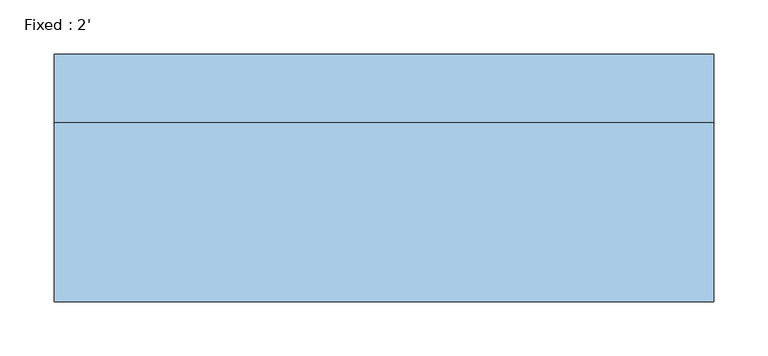
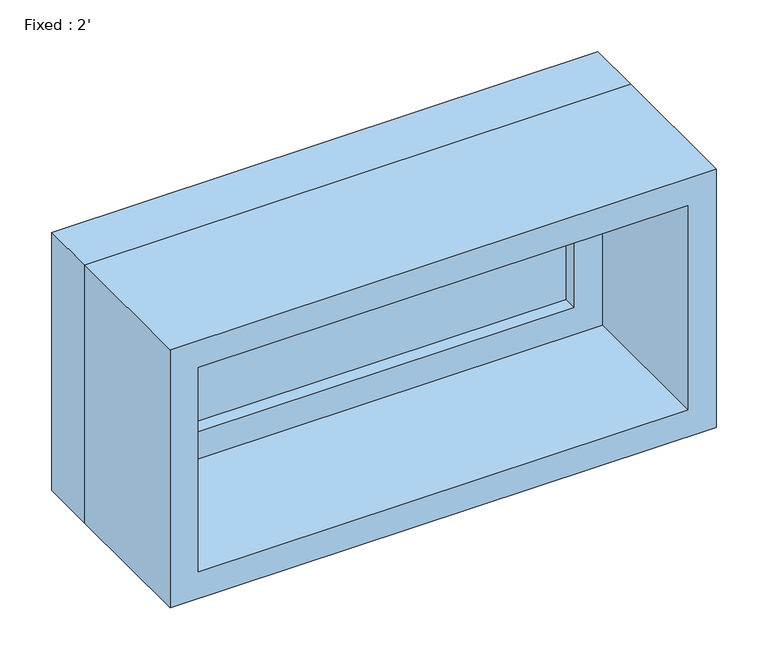
"""IFC4 building model written with IfcOpenShell, lengths in millimetres: window geometry, Fixed : 2'."""

from ifc_helpers import new_model, si_unit, frame, origin, place, context, project, spatial, polyline, outline, extrude, source, transform, mapped, element, save


def fixed_2_8c8825d0(model_context):
    return source(origin(), model_context, "Body", "SweptSolid", [
        extrude(outline(polyline([(203.2, 66.675), (-279.4, 66.675), (-279.4, 79.375), (203.2, 79.375), (203.2, 66.675)])), frame((0.0, 0.0, 977.9), z_axis=(0.0, 0.0, 1.0), x_axis=(1.0, 0.0, 0.0)), (0.0, 0.0, 1.0), 177.8),
        extrude(outline(polyline([(1200.15, -323.85), (933.45, -323.85), (933.45, 247.65), (1200.15, 247.65), (1200.15, -323.85)]), holes=[polyline([(1155.7, -279.4), (1155.7, 203.2), (977.9, 203.2), (977.9, -279.4), (1155.7, -279.4)])]), frame((0.0, 50.8, 0.0), z_axis=(0.0, 1.0, 0.0), x_axis=(0.0, 0.0, 1.0)), (0.0, 0.0, 1.0), 44.45),
        extrude(outline(polyline([(1219.2, -342.9), (914.4, -342.9), (914.4, 266.7), (1219.2, 266.7), (1219.2, -342.9)]), holes=[polyline([(1187.45, -311.15), (1187.45, 234.95), (946.15, 234.95), (946.15, -311.15), (1187.45, -311.15)])]), frame((0.0, -114.3, 0.0), z_axis=(0.0, 1.0, 0.0), x_axis=(0.0, 0.0, 1.0)), (0.0, 0.0, 1.0), 165.1),
        extrude(outline(polyline([(1219.2, 266.7), (1219.2, -342.9), (914.4, -342.9), (914.4, 266.7), (1219.2, 266.7)]), holes=[polyline([(1200.15, 247.65), (933.45, 247.65), (933.45, -323.85), (1200.15, -323.85), (1200.15, 247.65)])]), frame((0.0, 50.8, 0.0), z_axis=(0.0, 1.0, 0.0), x_axis=(0.0, 0.0, 1.0)), (0.0, 0.0, 1.0), 63.5),
    ])


if __name__ == "__main__":
    model = new_model("IFC4")
    model_context = context("Model", 3, world=origin())
    ifc_project = project(units=[si_unit("LENGTHUNIT", "METRE", prefix="MILLI")], contexts=[model_context])
    site = spatial("IfcSite", under=ifc_project)
    building = spatial("IfcBuilding", under=site)
    placement = place(None, origin())
    fixed_2_shape = fixed_2_8c8825d0(model_context)
    element("IfcWindow", 1, ObjectType="Fixed : 2'", at=placement, inside=building, context=model_context, shape_type="MappedRepresentation", body=[
        mapped(fixed_2_shape, transform((0.0, 0.0, 0.0), x_axis=(1.0, 0.0, 0.0), y_axis=(0.0, 1.0, 0.0), z_axis=(0.0, 0.0, 1.0))),
    ])
    save(model, "model.ifc")

# Revit data of these elements
# Type "Fixed : 2'"
#   Type Mark = "22"
#   Construction Type Id = "GSP4R"
#   Assembly Code = "B2020100"
#   Analytic Construction = "1/8 in Pilkington single glazing"
#   Visual Light Transmittance = 0.9
#   Solar Heat Gain Coefficient = 0.78
#   Heat Transfer Coefficient (U) = 0.6496 BTU/(h·ft²·°F)
#   Height = 1' - 0"
#   Default Sill Height = 3' - 0"
#   Width = 2' - 0"
#   Window Inset = 0' - 0 3/4"
#   Define Thermal Properties by = 1
#   Glass Pane Material = Glass
#   Sash Material = Sash
#   Wall Closure = (empty or 0)
# Element 1 (IfcWindow, "Fixed : 2'")
#   Materials on its faces: "Sash", "Glass"
# Materials
#   "Glass": class "Glass", colour RGB 0 128 192, transparency 0.75, Description = "Soda Lime Glass", Cost = 0
#   "Sash": class "Wood", colour RGB 224 178 126, transparency 0, Cost = 0
